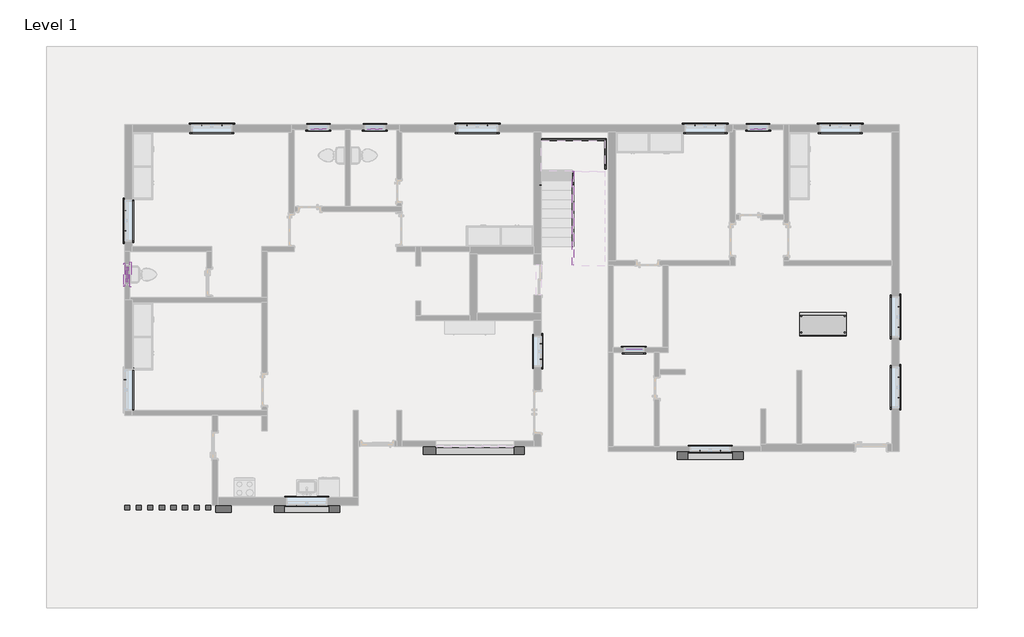
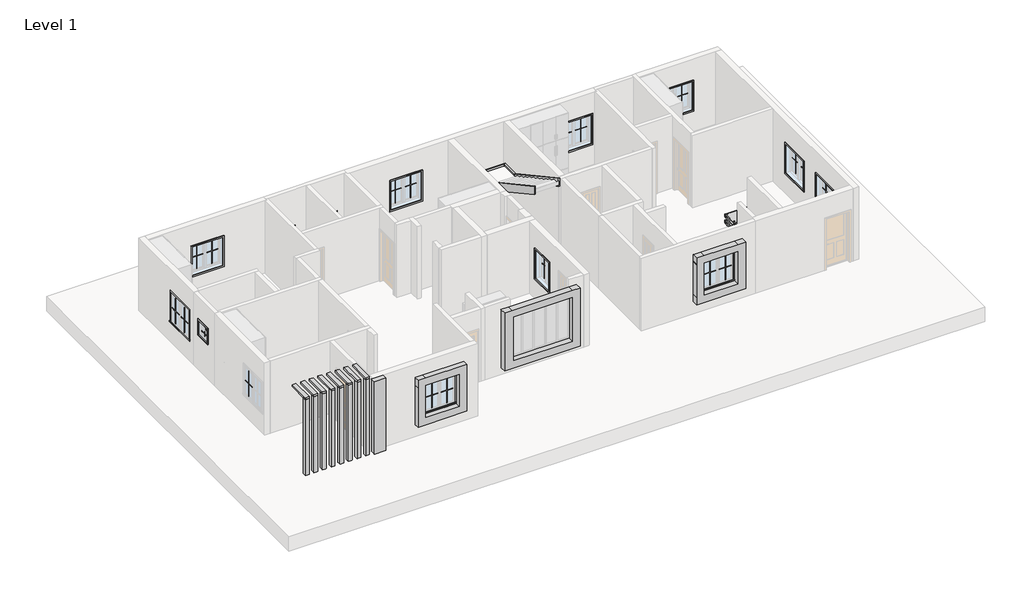
# One storey, part 3 of 3: 81 proxies, 7 members.
"""IFC4 building model written with IfcOpenShell, lengths in millimetres."""

from ifc_helpers import new_model, si_unit, frame, origin, place, context, project, spatial, polyline, outline, extrude, faceted_brep, transform, mapped, element, save
from components import generic_models_1_generic_models_1_a0d4ce11, generic_models_12_generic_models_1_bdc4cd0d, generic_models_13_generic_models_1_8ceb580d, generic_models_14_generic_models_1_67c994ca, generic_models_16_generic_models_16_6386461c, generic_models_17_generic_models_17_b8611751, generic_models_18_generic_models_18_97eb84db, generic_models_19_generic_models_19_60db133f, generic_models_2_generic_models_1_277b538b, generic_models_3_generic_models_1_ed787108, generic_models_4_generic_models_1_fab6a1cf, generic_models_5_generic_models_1_4439abc4, generic_models_6_generic_models_1_d5b3bf35, generic_models_7_generic_models_1_55103d6f, generic_models_8_generic_models_1_2d490598, modern_coffee_table_17989_modern_coffee_table_17989_d3a860c8, muntin_pattern_2x2_muntin_pattern_2x2_4dfeb3f3, muntin_pattern_2x2_muntin_pattern_2x2_e852a7e4, muntin_pattern_2x2_muntin_pattern_2x2_1acec82f, muntin_pattern_2x2_muntin_pattern_2x2_43d02eee, muntin_pattern_2x2_muntin_pattern_2x2_d17a704b, trim_window_exterior_flat_with_sill_7cfdd449, trim_window_exterior_flat_with_sill_e4b28ec3, trim_window_exterior_flat_with_sill_79c463f4, trim_window_interior_flat_picture_frame_f1e0b15b, trim_window_interior_flat_picture_frame_39ff4276, trim_window_interior_flat_picture_frame_0477b583

model = new_model("IFC4")

# Units and contexts
model_context = context("Model", 3, world=origin())
ifc_project = project(units=[si_unit("LENGTHUNIT", "METRE", prefix="MILLI")], contexts=[model_context])

# Site, building, storey
site = spatial("IfcSite", under=ifc_project)
building = spatial("IfcBuilding", under=site)
storey = spatial("IfcBuildingStorey", under=building, Name="Level 1", Elevation=0.0)

# Proxies
placement = place(None, origin())
generic_models_1_generic_models_1_shape = generic_models_1_generic_models_1_a0d4ce11(model_context)
element("IfcBuildingElementProxy", 1, Name="Generic Models 1 : Generic Models 1", ObjectType="Generic Models 1 : Generic Models 1", at=placement, inside=storey, context=model_context, shape_type="MappedRepresentation", body=[
    mapped(generic_models_1_generic_models_1_shape, transform((0.0, 0.0, 0.0), x_axis=(1.0, 0.0, 0.0), y_axis=(0.0, 1.0, 0.0), z_axis=(0.0, 0.0, 1.0))),
])
element("IfcBuildingElementProxy", 2, Name="Generic Models 10 : Generic Models 1", ObjectType="Generic Models 10 : Generic Models 1", at=placement, inside=storey, context=model_context, shape_type="MappedRepresentation", body=[
    mapped(generic_models_1_generic_models_1_shape, transform((0.0, 0.0, 0.0), x_axis=(1.0, 0.0, 0.0), y_axis=(0.0, 1.0, 0.0), z_axis=(0.0, 0.0, 1.0))),
])
element("IfcBuildingElementProxy", 3, Name="Generic Models 11 : Generic Models 1", ObjectType="Generic Models 11 : Generic Models 1", at=placement, inside=storey, context=model_context, shape_type="MappedRepresentation", body=[
    mapped(generic_models_1_generic_models_1_shape, transform((0.0, 0.0, 0.0), x_axis=(1.0, 0.0, 0.0), y_axis=(0.0, 1.0, 0.0), z_axis=(0.0, 0.0, 1.0))),
])
generic_models_12_generic_models_1_shape = generic_models_12_generic_models_1_bdc4cd0d(model_context)
element("IfcBuildingElementProxy", 4, Name="Generic Models 12 : Generic Models 1", ObjectType="Generic Models 12 : Generic Models 1", at=placement, inside=storey, context=model_context, shape_type="MappedRepresentation", body=[
    mapped(generic_models_12_generic_models_1_shape, transform((0.0, 0.0, 0.0), x_axis=(1.0, 0.0, 0.0), y_axis=(0.0, 1.0, 0.0), z_axis=(0.0, 0.0, 1.0))),
])
generic_models_13_generic_models_1_shape = generic_models_13_generic_models_1_8ceb580d(model_context)
element("IfcBuildingElementProxy", 5, Name="Generic Models 13 : Generic Models 1", ObjectType="Generic Models 13 : Generic Models 1", at=placement, inside=storey, context=model_context, shape_type="MappedRepresentation", body=[
    mapped(generic_models_13_generic_models_1_shape, transform((0.0, 0.0, 0.0), x_axis=(1.0, 0.0, 0.0), y_axis=(0.0, 1.0, 0.0), z_axis=(0.0, 0.0, 1.0))),
])
generic_models_14_generic_models_1_shape = generic_models_14_generic_models_1_67c994ca(model_context)
element("IfcBuildingElementProxy", 6, Name="Generic Models 14 : Generic Models 1", ObjectType="Generic Models 14 : Generic Models 1", at=placement, inside=storey, context=model_context, shape_type="MappedRepresentation", body=[
    mapped(generic_models_14_generic_models_1_shape, transform((0.0, 0.0, 0.0), x_axis=(1.0, 0.0, 0.0), y_axis=(0.0, 1.0, 0.0), z_axis=(0.0, 0.0, 1.0))),
])
generic_models_16_generic_models_16_shape = generic_models_16_generic_models_16_6386461c(model_context)
element("IfcBuildingElementProxy", 7, Name="Generic Models 16 : Generic Models 16", ObjectType="Generic Models 16 : Generic Models 16", at=placement, inside=storey, context=model_context, shape_type="MappedRepresentation", body=[
    mapped(generic_models_16_generic_models_16_shape, transform((0.0, 0.0, 0.0), x_axis=(1.0, 0.0, 0.0), y_axis=(0.0, 1.0, 0.0), z_axis=(0.0, 0.0, 1.0))),
])
generic_models_17_generic_models_17_shape = generic_models_17_generic_models_17_b8611751(model_context)
element("IfcBuildingElementProxy", 8, Name="Generic Models 17 : Generic Models 17", ObjectType="Generic Models 17 : Generic Models 17", at=placement, inside=storey, context=model_context, shape_type="MappedRepresentation", body=[
    mapped(generic_models_17_generic_models_17_shape, transform((0.0, 0.0, 0.0), x_axis=(1.0, 0.0, 0.0), y_axis=(0.0, 1.0, 0.0), z_axis=(0.0, 0.0, 1.0))),
])
generic_models_18_generic_models_18_shape = generic_models_18_generic_models_18_97eb84db(model_context)
element("IfcBuildingElementProxy", 9, Name="Generic Models 18 : Generic Models 18", ObjectType="Generic Models 18 : Generic Models 18", at=placement, inside=storey, context=model_context, shape_type="MappedRepresentation", body=[
    mapped(generic_models_18_generic_models_18_shape, transform((0.0, 0.0, 0.0), x_axis=(1.0, 0.0, 0.0), y_axis=(0.0, 1.0, 0.0), z_axis=(0.0, 0.0, 1.0))),
])
generic_models_19_generic_models_19_shape = generic_models_19_generic_models_19_60db133f(model_context)
element("IfcBuildingElementProxy", 10, Name="Generic Models 19 : Generic Models 19", ObjectType="Generic Models 19 : Generic Models 19", at=placement, inside=storey, context=model_context, shape_type="MappedRepresentation", body=[
    mapped(generic_models_19_generic_models_19_shape, transform((0.0, 0.0, 0.0), x_axis=(1.0, 0.0, 0.0), y_axis=(0.0, 1.0, 0.0), z_axis=(0.0, 0.0, 1.0))),
])
generic_models_2_generic_models_1_shape = generic_models_2_generic_models_1_277b538b(model_context)
element("IfcBuildingElementProxy", 11, Name="Generic Models 2 : Generic Models 1", ObjectType="Generic Models 2 : Generic Models 1", at=placement, inside=storey, context=model_context, shape_type="MappedRepresentation", body=[
    mapped(generic_models_2_generic_models_1_shape, transform((0.0, 0.0, 0.0), x_axis=(1.0, 0.0, 0.0), y_axis=(0.0, 1.0, 0.0), z_axis=(0.0, 0.0, 1.0))),
])
generic_models_3_generic_models_1_shape = generic_models_3_generic_models_1_ed787108(model_context)
element("IfcBuildingElementProxy", 12, Name="Generic Models 3 : Generic Models 1", ObjectType="Generic Models 3 : Generic Models 1", at=placement, inside=storey, context=model_context, shape_type="MappedRepresentation", body=[
    mapped(generic_models_3_generic_models_1_shape, transform((0.0, 0.0, 0.0), x_axis=(1.0, 0.0, 0.0), y_axis=(0.0, 1.0, 0.0), z_axis=(0.0, 0.0, 1.0))),
])
generic_models_4_generic_models_1_shape = generic_models_4_generic_models_1_fab6a1cf(model_context)
element("IfcBuildingElementProxy", 13, Name="Generic Models 4 : Generic Models 1", ObjectType="Generic Models 4 : Generic Models 1", at=placement, inside=storey, context=model_context, shape_type="MappedRepresentation", body=[
    mapped(generic_models_4_generic_models_1_shape, transform((0.0, 0.0, 0.0), x_axis=(1.0, 0.0, 0.0), y_axis=(0.0, 1.0, 0.0), z_axis=(0.0, 0.0, 1.0))),
])
generic_models_5_generic_models_1_shape = generic_models_5_generic_models_1_4439abc4(model_context)
element("IfcBuildingElementProxy", 14, Name="Generic Models 5 : Generic Models 1", ObjectType="Generic Models 5 : Generic Models 1", at=placement, inside=storey, context=model_context, shape_type="MappedRepresentation", body=[
    mapped(generic_models_5_generic_models_1_shape, transform((0.0, 0.0, 0.0), x_axis=(1.0, 0.0, 0.0), y_axis=(0.0, 1.0, 0.0), z_axis=(0.0, 0.0, 1.0))),
])
generic_models_6_generic_models_1_shape = generic_models_6_generic_models_1_d5b3bf35(model_context)
element("IfcBuildingElementProxy", 15, Name="Generic Models 6 : Generic Models 1", ObjectType="Generic Models 6 : Generic Models 1", at=placement, inside=storey, context=model_context, shape_type="MappedRepresentation", body=[
    mapped(generic_models_6_generic_models_1_shape, transform((0.0, 0.0, 0.0), x_axis=(1.0, 0.0, 0.0), y_axis=(0.0, 1.0, 0.0), z_axis=(0.0, 0.0, 1.0))),
])
generic_models_7_generic_models_1_shape = generic_models_7_generic_models_1_55103d6f(model_context)
element("IfcBuildingElementProxy", 16, Name="Generic Models 7 : Generic Models 1", ObjectType="Generic Models 7 : Generic Models 1", at=placement, inside=storey, context=model_context, shape_type="MappedRepresentation", body=[
    mapped(generic_models_7_generic_models_1_shape, transform((0.0, 0.0, 0.0), x_axis=(1.0, 0.0, 0.0), y_axis=(0.0, 1.0, 0.0), z_axis=(0.0, 0.0, 1.0))),
])
generic_models_8_generic_models_1_shape = generic_models_8_generic_models_1_2d490598(model_context)
element("IfcBuildingElementProxy", 17, Name="Generic Models 8 : Generic Models 1", ObjectType="Generic Models 8 : Generic Models 1", at=placement, inside=storey, context=model_context, shape_type="MappedRepresentation", body=[
    mapped(generic_models_8_generic_models_1_shape, transform((0.0, 0.0, 0.0), x_axis=(1.0, 0.0, 0.0), y_axis=(0.0, 1.0, 0.0), z_axis=(0.0, 0.0, 1.0))),
])
element("IfcBuildingElementProxy", 18, Name="Generic Models 9 : Generic Models 1", ObjectType="Generic Models 9 : Generic Models 1", at=placement, inside=storey, context=model_context, shape_type="MappedRepresentation", body=[
    mapped(generic_models_1_generic_models_1_shape, transform((0.0, 0.0, 0.0), x_axis=(1.0, 0.0, 0.0), y_axis=(0.0, 1.0, 0.0), z_axis=(0.0, 0.0, 1.0))),
])
modern_coffee_table_17989_modern_coffee_table_17989_shape = modern_coffee_table_17989_modern_coffee_table_17989_d3a860c8(model_context)
element("IfcBuildingElementProxy", 19, Name="Modern_Coffee_Table_17989 : Modern_Coffee_Table_17989", ObjectType="Modern_Coffee_Table_17989 : Modern_Coffee_Table_17989", at=placement, inside=storey, context=model_context, shape_type="MappedRepresentation", body=[
    mapped(modern_coffee_table_17989_modern_coffee_table_17989_shape, transform((8876.5549644, 263.8114998, 0.0), x_axis=(1.0, 0.0, 0.0), y_axis=(0.0, 1.0, 0.0), z_axis=(0.0, 0.0, 1.0))),
])
muntin_pattern_2x2_muntin_pattern_2x2_shape = muntin_pattern_2x2_muntin_pattern_2x2_4dfeb3f3(model_context)
element("IfcBuildingElementProxy", 20, Name="Muntin Pattern_2x2 : Muntin Pattern_2x2", ObjectType="Muntin Pattern_2x2 : Muntin Pattern_2x2", at=placement, inside=storey, context=model_context, shape_type="MappedRepresentation", body=[
    mapped(muntin_pattern_2x2_muntin_pattern_2x2_shape, transform((-9812.5661806, 5834.4476898, 984.25), x_axis=(1.0, 0.0, 0.0), y_axis=(0.0, 1.0, 0.0), z_axis=(0.0, 0.0, 1.0))),
])
element("IfcBuildingElementProxy", 21, Name="Muntin Pattern_2x2 : Muntin Pattern_2x2", ObjectType="Muntin Pattern_2x2 : Muntin Pattern_2x2", at=placement, inside=storey, context=model_context, shape_type="MappedRepresentation", body=[
    mapped(muntin_pattern_2x2_muntin_pattern_2x2_shape, transform((-1925.8661806, 5834.4476898, 984.25), x_axis=(1.0, 0.0, 0.0), y_axis=(0.0, 1.0, 0.0), z_axis=(0.0, 0.0, 1.0))),
])
element("IfcBuildingElementProxy", 22, Name="Muntin Pattern_2x2 : Muntin Pattern_2x2", ObjectType="Muntin Pattern_2x2 : Muntin Pattern_2x2", at=placement, inside=storey, context=model_context, shape_type="MappedRepresentation", body=[
    mapped(muntin_pattern_2x2_muntin_pattern_2x2_shape, transform((4843.2338194, 5834.4476898, 984.25), x_axis=(1.0, 0.0, 0.0), y_axis=(0.0, 1.0, 0.0), z_axis=(0.0, 0.0, 1.0))),
])
element("IfcBuildingElementProxy", 23, Name="Muntin Pattern_2x2 : Muntin Pattern_2x2", ObjectType="Muntin Pattern_2x2 : Muntin Pattern_2x2", at=placement, inside=storey, context=model_context, shape_type="MappedRepresentation", body=[
    mapped(muntin_pattern_2x2_muntin_pattern_2x2_shape, transform((8856.4338194, 5834.4476898, 984.25), x_axis=(1.0, 0.0, 0.0), y_axis=(0.0, 1.0, 0.0), z_axis=(0.0, 0.0, 1.0))),
])
element("IfcBuildingElementProxy", 24, Name="Muntin Pattern_2x2 : Muntin Pattern_2x2", ObjectType="Muntin Pattern_2x2 : Muntin Pattern_2x2", at=placement, inside=storey, context=model_context, shape_type="MappedRepresentation", body=[
    mapped(muntin_pattern_2x2_muntin_pattern_2x2_shape, transform((10902.7213194, 432.1851898, 984.25), x_axis=(0.0, -1.0, 0.0), y_axis=(1.0, 0.0, 0.0), z_axis=(0.0, 0.0, 1.0))),
])
element("IfcBuildingElementProxy", 25, Name="Muntin Pattern_2x2 : Muntin Pattern_2x2", ObjectType="Muntin Pattern_2x2 : Muntin Pattern_2x2", at=placement, inside=storey, context=model_context, shape_type="MappedRepresentation", body=[
    mapped(muntin_pattern_2x2_muntin_pattern_2x2_shape, transform((10902.7213194, -1663.3148102, 984.25), x_axis=(0.0, -1.0, 0.0), y_axis=(1.0, 0.0, 0.0), z_axis=(0.0, 0.0, 1.0))),
])
element("IfcBuildingElementProxy", 26, Name="Muntin Pattern_2x2 : Muntin Pattern_2x2", ObjectType="Muntin Pattern_2x2 : Muntin Pattern_2x2", at=placement, inside=storey, context=model_context, shape_type="MappedRepresentation", body=[
    mapped(muntin_pattern_2x2_muntin_pattern_2x2_shape, transform((5595.7088194, -3862.0023102, 984.25), x_axis=(-1.0, 0.0, 0.0), y_axis=(0.0, -1.0, 0.0), z_axis=(0.0, 0.0, 1.0))),
])
element("IfcBuildingElementProxy", 27, Name="Muntin Pattern_2x2 : Muntin Pattern_2x2", ObjectType="Muntin Pattern_2x2 : Muntin Pattern_2x2", at=placement, inside=storey, context=model_context, shape_type="MappedRepresentation", body=[
    mapped(muntin_pattern_2x2_muntin_pattern_2x2_shape, transform((-12090.6286806, 2683.2601898, 984.25), x_axis=(0.0, 1.0, 0.0), y_axis=(-1.0, 0.0, 0.0), z_axis=(0.0, 0.0, 1.0))),
])
element("IfcBuildingElementProxy", 28, Name="Muntin Pattern_2x2 : Muntin Pattern_2x2", ObjectType="Muntin Pattern_2x2 : Muntin Pattern_2x2", at=placement, inside=storey, context=model_context, shape_type="MappedRepresentation", body=[
    mapped(muntin_pattern_2x2_muntin_pattern_2x2_shape, transform((-6386.7411806, -5462.2023102, 984.25), x_axis=(-1.0, 0.0, 0.0), y_axis=(0.0, -1.0, 0.0), z_axis=(0.0, 0.0, 1.0))),
])
muntin_pattern_2x2_muntin_pattern_2x2_2_shape = muntin_pattern_2x2_muntin_pattern_2x2_e852a7e4(model_context)
element("IfcBuildingElementProxy", 29, Name="Muntin Pattern_2x2 : Muntin Pattern_2x2", ObjectType="Muntin Pattern_2x2 : Muntin Pattern_2x2", at=placement, inside=storey, context=model_context, shape_type="MappedRepresentation", body=[
    mapped(muntin_pattern_2x2_muntin_pattern_2x2_2_shape, transform((-9206.1411806, 5834.4476898, 984.25), x_axis=(-1.0, 0.0, 0.0), y_axis=(0.0, -1.0, 0.0), z_axis=(0.0, 0.0, 1.0))),
])
element("IfcBuildingElementProxy", 30, Name="Muntin Pattern_2x2 : Muntin Pattern_2x2", ObjectType="Muntin Pattern_2x2 : Muntin Pattern_2x2", at=placement, inside=storey, context=model_context, shape_type="MappedRepresentation", body=[
    mapped(muntin_pattern_2x2_muntin_pattern_2x2_2_shape, transform((-1319.4411806, 5834.4476898, 984.25), x_axis=(-1.0, 0.0, 0.0), y_axis=(0.0, -1.0, 0.0), z_axis=(0.0, 0.0, 1.0))),
])
element("IfcBuildingElementProxy", 31, Name="Muntin Pattern_2x2 : Muntin Pattern_2x2", ObjectType="Muntin Pattern_2x2 : Muntin Pattern_2x2", at=placement, inside=storey, context=model_context, shape_type="MappedRepresentation", body=[
    mapped(muntin_pattern_2x2_muntin_pattern_2x2_2_shape, transform((5449.6588194, 5834.4476898, 984.25), x_axis=(-1.0, 0.0, 0.0), y_axis=(0.0, -1.0, 0.0), z_axis=(0.0, 0.0, 1.0))),
])
element("IfcBuildingElementProxy", 32, Name="Muntin Pattern_2x2 : Muntin Pattern_2x2", ObjectType="Muntin Pattern_2x2 : Muntin Pattern_2x2", at=placement, inside=storey, context=model_context, shape_type="MappedRepresentation", body=[
    mapped(muntin_pattern_2x2_muntin_pattern_2x2_2_shape, transform((9462.8588194, 5834.4476898, 984.25), x_axis=(-1.0, 0.0, 0.0), y_axis=(0.0, -1.0, 0.0), z_axis=(0.0, 0.0, 1.0))),
])
element("IfcBuildingElementProxy", 33, Name="Muntin Pattern_2x2 : Muntin Pattern_2x2", ObjectType="Muntin Pattern_2x2 : Muntin Pattern_2x2", at=placement, inside=storey, context=model_context, shape_type="MappedRepresentation", body=[
    mapped(muntin_pattern_2x2_muntin_pattern_2x2_2_shape, transform((10902.7213194, -174.2398102, 984.25), x_axis=(0.0, 1.0, 0.0), y_axis=(-1.0, 0.0, 0.0), z_axis=(0.0, 0.0, 1.0))),
])
element("IfcBuildingElementProxy", 34, Name="Muntin Pattern_2x2 : Muntin Pattern_2x2", ObjectType="Muntin Pattern_2x2 : Muntin Pattern_2x2", at=placement, inside=storey, context=model_context, shape_type="MappedRepresentation", body=[
    mapped(muntin_pattern_2x2_muntin_pattern_2x2_2_shape, transform((10902.7213194, -2269.7398102, 984.25), x_axis=(0.0, 1.0, 0.0), y_axis=(-1.0, 0.0, 0.0), z_axis=(0.0, 0.0, 1.0))),
])
element("IfcBuildingElementProxy", 35, Name="Muntin Pattern_2x2 : Muntin Pattern_2x2", ObjectType="Muntin Pattern_2x2 : Muntin Pattern_2x2", at=placement, inside=storey, context=model_context, shape_type="MappedRepresentation", body=[
    mapped(muntin_pattern_2x2_muntin_pattern_2x2_2_shape, transform((-12090.6286806, -1739.5148102, 984.25), x_axis=(0.0, -1.0, 0.0), y_axis=(1.0, 0.0, 0.0), z_axis=(0.0, 0.0, 1.0))),
])
element("IfcBuildingElementProxy", 36, Name="Muntin Pattern_2x2 : Muntin Pattern_2x2", ObjectType="Muntin Pattern_2x2 : Muntin Pattern_2x2", at=placement, inside=storey, context=model_context, shape_type="MappedRepresentation", body=[
    mapped(muntin_pattern_2x2_muntin_pattern_2x2_2_shape, transform((4989.2838194, -3862.0023102, 984.25), x_axis=(1.0, 0.0, 0.0), y_axis=(0.0, 1.0, 0.0), z_axis=(0.0, 0.0, 1.0))),
])
element("IfcBuildingElementProxy", 37, Name="Muntin Pattern_2x2 : Muntin Pattern_2x2", ObjectType="Muntin Pattern_2x2 : Muntin Pattern_2x2", at=placement, inside=storey, context=model_context, shape_type="MappedRepresentation", body=[
    mapped(muntin_pattern_2x2_muntin_pattern_2x2_2_shape, transform((-12090.6286806, 3289.6851898, 984.25), x_axis=(0.0, -1.0, 0.0), y_axis=(1.0, 0.0, 0.0), z_axis=(0.0, 0.0, 1.0))),
])
element("IfcBuildingElementProxy", 38, Name="Muntin Pattern_2x2 : Muntin Pattern_2x2", ObjectType="Muntin Pattern_2x2 : Muntin Pattern_2x2", at=placement, inside=storey, context=model_context, shape_type="MappedRepresentation", body=[
    mapped(muntin_pattern_2x2_muntin_pattern_2x2_2_shape, transform((-6993.1661806, -5462.2023102, 984.25), x_axis=(1.0, 0.0, 0.0), y_axis=(0.0, 1.0, 0.0), z_axis=(0.0, 0.0, 1.0))),
])
muntin_pattern_2x2_muntin_pattern_2x2_3_shape = muntin_pattern_2x2_muntin_pattern_2x2_1acec82f(model_context)
element("IfcBuildingElementProxy", 39, Name="Muntin Pattern_2x2 : Muntin Pattern_2x2", ObjectType="Muntin Pattern_2x2 : Muntin Pattern_2x2", at=placement, inside=storey, context=model_context, shape_type="MappedRepresentation", body=[
    mapped(muntin_pattern_2x2_muntin_pattern_2x2_3_shape, transform((272.8213194, -672.7148102, 984.25), x_axis=(0.0, -1.0, 0.0), y_axis=(1.0, 0.0, 0.0), z_axis=(0.0, 0.0, 1.0))),
])
muntin_pattern_2x2_muntin_pattern_2x2_4_shape = muntin_pattern_2x2_muntin_pattern_2x2_43d02eee(model_context)
element("IfcBuildingElementProxy", 40, Name="Muntin Pattern_2x2 : Muntin Pattern_2x2", ObjectType="Muntin Pattern_2x2 : Muntin Pattern_2x2", at=placement, inside=storey, context=model_context, shape_type="MappedRepresentation", body=[
    mapped(muntin_pattern_2x2_muntin_pattern_2x2_4_shape, transform((272.8213194, -1126.7398102, 984.25), x_axis=(0.0, 1.0, 0.0), y_axis=(-1.0, 0.0, 0.0), z_axis=(0.0, 0.0, 1.0))),
])
muntin_pattern_2x2_muntin_pattern_2x2_5_shape = muntin_pattern_2x2_muntin_pattern_2x2_d17a704b(model_context)
element("IfcBuildingElementProxy", 41, Name="Muntin Pattern_2x2 : Muntin Pattern_2x2", ObjectType="Muntin Pattern_2x2 : Muntin Pattern_2x2", at=placement, inside=storey, context=model_context, shape_type="MappedRepresentation", body=[
    mapped(muntin_pattern_2x2_muntin_pattern_2x2_5_shape, transform((-11982.6786806, 1386.2726898, 1844.675), x_axis=(0.0, -1.0, 0.0), y_axis=(1.0, 0.0, 0.0), z_axis=(0.0, 0.0, 1.0))),
])
element("IfcBuildingElementProxy", 42, Name="Muntin Pattern_2x2 : Muntin Pattern_2x2", ObjectType="Muntin Pattern_2x2 : Muntin Pattern_2x2", at=placement, inside=storey, context=model_context, shape_type="MappedRepresentation", body=[
    mapped(muntin_pattern_2x2_muntin_pattern_2x2_5_shape, transform((-12027.1286806, 1386.2726898, 1600.2), x_axis=(0.0, -1.0, 0.0), y_axis=(1.0, 0.0, 0.0), z_axis=(0.0, 0.0, 1.0))),
])
element("IfcBuildingElementProxy", 43, Name="Muntin Pattern_2x2 : Muntin Pattern_2x2", ObjectType="Muntin Pattern_2x2 : Muntin Pattern_2x2", at=placement, inside=storey, context=model_context, shape_type="MappedRepresentation", body=[
    mapped(muntin_pattern_2x2_muntin_pattern_2x2_5_shape, transform((-6347.0536806, 5726.4976898, 1235.075), x_axis=(-1.0, 0.0, 0.0), y_axis=(0.0, -1.0, 0.0), z_axis=(0.0, 0.0, 1.0))),
])
element("IfcBuildingElementProxy", 44, Name="Muntin Pattern_2x2 : Muntin Pattern_2x2", ObjectType="Muntin Pattern_2x2 : Muntin Pattern_2x2", at=placement, inside=storey, context=model_context, shape_type="MappedRepresentation", body=[
    mapped(muntin_pattern_2x2_muntin_pattern_2x2_5_shape, transform((-6347.0536806, 5770.9476898, 990.6), x_axis=(-1.0, 0.0, 0.0), y_axis=(0.0, -1.0, 0.0), z_axis=(0.0, 0.0, 1.0))),
])
element("IfcBuildingElementProxy", 45, Name="Muntin Pattern_2x2 : Muntin Pattern_2x2", ObjectType="Muntin Pattern_2x2 : Muntin Pattern_2x2", at=placement, inside=storey, context=model_context, shape_type="MappedRepresentation", body=[
    mapped(muntin_pattern_2x2_muntin_pattern_2x2_5_shape, transform((-4670.6536806, 5726.4976898, 1235.075), x_axis=(-1.0, 0.0, 0.0), y_axis=(0.0, -1.0, 0.0), z_axis=(0.0, 0.0, 1.0))),
])
element("IfcBuildingElementProxy", 46, Name="Muntin Pattern_2x2 : Muntin Pattern_2x2", ObjectType="Muntin Pattern_2x2 : Muntin Pattern_2x2", at=placement, inside=storey, context=model_context, shape_type="MappedRepresentation", body=[
    mapped(muntin_pattern_2x2_muntin_pattern_2x2_5_shape, transform((-4670.6536806, 5770.9476898, 990.6), x_axis=(-1.0, 0.0, 0.0), y_axis=(0.0, -1.0, 0.0), z_axis=(0.0, 0.0, 1.0))),
])
element("IfcBuildingElementProxy", 47, Name="Muntin Pattern_2x2 : Muntin Pattern_2x2", ObjectType="Muntin Pattern_2x2 : Muntin Pattern_2x2", at=placement, inside=storey, context=model_context, shape_type="MappedRepresentation", body=[
    mapped(muntin_pattern_2x2_muntin_pattern_2x2_5_shape, transform((6721.2463194, 5726.4976898, 1235.075), x_axis=(-1.0, 0.0, 0.0), y_axis=(0.0, -1.0, 0.0), z_axis=(0.0, 0.0, 1.0))),
])
element("IfcBuildingElementProxy", 48, Name="Muntin Pattern_2x2 : Muntin Pattern_2x2", ObjectType="Muntin Pattern_2x2 : Muntin Pattern_2x2", at=placement, inside=storey, context=model_context, shape_type="MappedRepresentation", body=[
    mapped(muntin_pattern_2x2_muntin_pattern_2x2_5_shape, transform((6721.2463194, 5770.9476898, 990.6), x_axis=(-1.0, 0.0, 0.0), y_axis=(0.0, -1.0, 0.0), z_axis=(0.0, 0.0, 1.0))),
])
element("IfcBuildingElementProxy", 49, Name="Muntin Pattern_2x2 : Muntin Pattern_2x2", ObjectType="Muntin Pattern_2x2 : Muntin Pattern_2x2", at=placement, inside=storey, context=model_context, shape_type="MappedRepresentation", body=[
    mapped(muntin_pattern_2x2_muntin_pattern_2x2_5_shape, transform((3025.5463194, -820.3523102, 1235.075), x_axis=(1.0, 0.0, 0.0), y_axis=(0.0, 1.0, 0.0), z_axis=(0.0, 0.0, 1.0))),
])
element("IfcBuildingElementProxy", 50, Name="Muntin Pattern_2x2 : Muntin Pattern_2x2", ObjectType="Muntin Pattern_2x2 : Muntin Pattern_2x2", at=placement, inside=storey, context=model_context, shape_type="MappedRepresentation", body=[
    mapped(muntin_pattern_2x2_muntin_pattern_2x2_5_shape, transform((3025.5463194, -864.8023102, 990.6), x_axis=(1.0, 0.0, 0.0), y_axis=(0.0, 1.0, 0.0), z_axis=(0.0, 0.0, 1.0))),
])
trim_window_exterior_flat_with_sill_shape = trim_window_exterior_flat_with_sill_7cfdd449(model_context)
element("IfcBuildingElementProxy", 51, Name="Trim-Window-Exterior-Flat : with Sill", ObjectType="Trim-Window-Exterior-Flat : with Sill", at=placement, inside=storey, context=model_context, shape_type="MappedRepresentation", body=[
    mapped(trim_window_exterior_flat_with_sill_shape, transform((-9509.3536806, 5843.9726898, 2133.6), x_axis=(-1.0, 0.0, 0.0), y_axis=(0.0, 0.0, 1.0), z_axis=(0.0, 1.0, 0.0))),
])
element("IfcBuildingElementProxy", 52, Name="Trim-Window-Exterior-Flat : with Sill", ObjectType="Trim-Window-Exterior-Flat : with Sill", at=placement, inside=storey, context=model_context, shape_type="MappedRepresentation", body=[
    mapped(trim_window_exterior_flat_with_sill_shape, transform((-1622.6536806, 5843.9726898, 2133.6), x_axis=(-1.0, 0.0, 0.0), y_axis=(0.0, 0.0, 1.0), z_axis=(0.0, 1.0, 0.0))),
])
element("IfcBuildingElementProxy", 53, Name="Trim-Window-Exterior-Flat : with Sill", ObjectType="Trim-Window-Exterior-Flat : with Sill", at=placement, inside=storey, context=model_context, shape_type="MappedRepresentation", body=[
    mapped(trim_window_exterior_flat_with_sill_shape, transform((5146.4463194, 5843.9726898, 2133.6), x_axis=(-1.0, 0.0, 0.0), y_axis=(0.0, 0.0, 1.0), z_axis=(0.0, 1.0, 0.0))),
])
element("IfcBuildingElementProxy", 54, Name="Trim-Window-Exterior-Flat : with Sill", ObjectType="Trim-Window-Exterior-Flat : with Sill", at=placement, inside=storey, context=model_context, shape_type="MappedRepresentation", body=[
    mapped(trim_window_exterior_flat_with_sill_shape, transform((9159.6463194, 5843.9726898, 2133.6), x_axis=(-1.0, 0.0, 0.0), y_axis=(0.0, 0.0, 1.0), z_axis=(0.0, 1.0, 0.0))),
])
element("IfcBuildingElementProxy", 55, Name="Trim-Window-Exterior-Flat : with Sill", ObjectType="Trim-Window-Exterior-Flat : with Sill", at=placement, inside=storey, context=model_context, shape_type="MappedRepresentation", body=[
    mapped(trim_window_exterior_flat_with_sill_shape, transform((10912.2463194, 128.9726898, 2133.6), x_axis=(0.0, 1.0, 0.0), y_axis=(0.0, 0.0, 1.0), z_axis=(1.0, 0.0, 0.0))),
])
element("IfcBuildingElementProxy", 56, Name="Trim-Window-Exterior-Flat : with Sill", ObjectType="Trim-Window-Exterior-Flat : with Sill", at=placement, inside=storey, context=model_context, shape_type="MappedRepresentation", body=[
    mapped(trim_window_exterior_flat_with_sill_shape, transform((10912.2463194, -1966.5273102, 2133.6), x_axis=(0.0, 1.0, 0.0), y_axis=(0.0, 0.0, 1.0), z_axis=(1.0, 0.0, 0.0))),
])
element("IfcBuildingElementProxy", 57, Name="Trim-Window-Exterior-Flat : with Sill", ObjectType="Trim-Window-Exterior-Flat : with Sill", at=placement, inside=storey, context=model_context, shape_type="MappedRepresentation", body=[
    mapped(trim_window_exterior_flat_with_sill_shape, transform((5292.4963194, -3871.5273102, 2133.6), x_axis=(1.0, 0.0, 0.0), y_axis=(0.0, 0.0, 1.0), z_axis=(0.0, -1.0, 0.0))),
])
element("IfcBuildingElementProxy", 58, Name="Trim-Window-Exterior-Flat : with Sill", ObjectType="Trim-Window-Exterior-Flat : with Sill", at=placement, inside=storey, context=model_context, shape_type="MappedRepresentation", body=[
    mapped(trim_window_exterior_flat_with_sill_shape, transform((-12100.1536806, 2986.4726898, 2133.6), x_axis=(0.0, -1.0, 0.0), y_axis=(0.0, 0.0, 1.0), z_axis=(-1.0, 0.0, 0.0))),
])
element("IfcBuildingElementProxy", 59, Name="Trim-Window-Exterior-Flat : with Sill", ObjectType="Trim-Window-Exterior-Flat : with Sill", at=placement, inside=storey, context=model_context, shape_type="MappedRepresentation", body=[
    mapped(trim_window_exterior_flat_with_sill_shape, transform((-6689.9536806, -5471.7273102, 2133.6), x_axis=(1.0, 0.0, 0.0), y_axis=(0.0, 0.0, 1.0), z_axis=(0.0, -1.0, 0.0))),
])
trim_window_exterior_flat_with_sill_2_shape = trim_window_exterior_flat_with_sill_e4b28ec3(model_context)
element("IfcBuildingElementProxy", 60, Name="Trim-Window-Exterior-Flat : with Sill", ObjectType="Trim-Window-Exterior-Flat : with Sill", at=placement, inside=storey, context=model_context, shape_type="MappedRepresentation", body=[
    mapped(trim_window_exterior_flat_with_sill_2_shape, transform((282.3463194, -899.7273102, 2133.6), x_axis=(0.0, 1.0, 0.0), y_axis=(0.0, 0.0, 1.0), z_axis=(1.0, 0.0, 0.0))),
])
trim_window_exterior_flat_with_sill_3_shape = trim_window_exterior_flat_with_sill_79c463f4(model_context)
element("IfcBuildingElementProxy", 61, Name="Trim-Window-Exterior-Flat : with Sill", ObjectType="Trim-Window-Exterior-Flat : with Sill", at=placement, inside=storey, context=model_context, shape_type="MappedRepresentation", body=[
    mapped(trim_window_exterior_flat_with_sill_3_shape, transform((-11947.7536806, 1386.2726898, 2120.9), x_axis=(0.0, 1.0, 0.0), y_axis=(0.0, 0.0, 1.0), z_axis=(1.0, 0.0, 0.0))),
])
element("IfcBuildingElementProxy", 62, Name="Trim-Window-Exterior-Flat : with Sill", ObjectType="Trim-Window-Exterior-Flat : with Sill", at=placement, inside=storey, context=model_context, shape_type="MappedRepresentation", body=[
    mapped(trim_window_exterior_flat_with_sill_3_shape, transform((-6347.0536806, 5691.5726898, 1511.3), x_axis=(1.0, 0.0, 0.0), y_axis=(0.0, 0.0, 1.0), z_axis=(0.0, -1.0, 0.0))),
])
element("IfcBuildingElementProxy", 63, Name="Trim-Window-Exterior-Flat : with Sill", ObjectType="Trim-Window-Exterior-Flat : with Sill", at=placement, inside=storey, context=model_context, shape_type="MappedRepresentation", body=[
    mapped(trim_window_exterior_flat_with_sill_3_shape, transform((-4670.6536806, 5691.5726898, 1511.3), x_axis=(1.0, 0.0, 0.0), y_axis=(0.0, 0.0, 1.0), z_axis=(0.0, -1.0, 0.0))),
])
element("IfcBuildingElementProxy", 64, Name="Trim-Window-Exterior-Flat : with Sill", ObjectType="Trim-Window-Exterior-Flat : with Sill", at=placement, inside=storey, context=model_context, shape_type="MappedRepresentation", body=[
    mapped(trim_window_exterior_flat_with_sill_3_shape, transform((6721.2463194, 5691.5726898, 1511.3), x_axis=(1.0, 0.0, 0.0), y_axis=(0.0, 0.0, 1.0), z_axis=(0.0, -1.0, 0.0))),
])
element("IfcBuildingElementProxy", 65, Name="Trim-Window-Exterior-Flat : with Sill", ObjectType="Trim-Window-Exterior-Flat : with Sill", at=placement, inside=storey, context=model_context, shape_type="MappedRepresentation", body=[
    mapped(trim_window_exterior_flat_with_sill_3_shape, transform((3025.5463194, -785.4273102, 1511.3), x_axis=(-1.0, 0.0, 0.0), y_axis=(0.0, 0.0, 1.0), z_axis=(0.0, 1.0, 0.0))),
])
trim_window_interior_flat_picture_frame_shape = trim_window_interior_flat_picture_frame_f1e0b15b(model_context)
element("IfcBuildingElementProxy", 66, Name="Trim-Window-Interior-Flat : Picture Frame", ObjectType="Trim-Window-Interior-Flat : Picture Frame", at=placement, inside=storey, context=model_context, shape_type="MappedRepresentation", body=[
    mapped(trim_window_interior_flat_picture_frame_shape, transform((-9509.3536806, 5615.3726898, 2133.6), x_axis=(1.0, 0.0, 0.0), y_axis=(0.0, 0.0, 1.0), z_axis=(0.0, -1.0, 0.0))),
])
element("IfcBuildingElementProxy", 67, Name="Trim-Window-Interior-Flat : Picture Frame", ObjectType="Trim-Window-Interior-Flat : Picture Frame", at=placement, inside=storey, context=model_context, shape_type="MappedRepresentation", body=[
    mapped(trim_window_interior_flat_picture_frame_shape, transform((-1622.6536806, 5615.3726898, 2133.6), x_axis=(1.0, 0.0, 0.0), y_axis=(0.0, 0.0, 1.0), z_axis=(0.0, -1.0, 0.0))),
])
element("IfcBuildingElementProxy", 68, Name="Trim-Window-Interior-Flat : Picture Frame", ObjectType="Trim-Window-Interior-Flat : Picture Frame", at=placement, inside=storey, context=model_context, shape_type="MappedRepresentation", body=[
    mapped(trim_window_interior_flat_picture_frame_shape, transform((5146.4463194, 5615.3726898, 2133.6), x_axis=(1.0, 0.0, 0.0), y_axis=(0.0, 0.0, 1.0), z_axis=(0.0, -1.0, 0.0))),
])
element("IfcBuildingElementProxy", 69, Name="Trim-Window-Interior-Flat : Picture Frame", ObjectType="Trim-Window-Interior-Flat : Picture Frame", at=placement, inside=storey, context=model_context, shape_type="MappedRepresentation", body=[
    mapped(trim_window_interior_flat_picture_frame_shape, transform((9159.6463194, 5615.3726898, 2133.6), x_axis=(1.0, 0.0, 0.0), y_axis=(0.0, 0.0, 1.0), z_axis=(0.0, -1.0, 0.0))),
])
element("IfcBuildingElementProxy", 70, Name="Trim-Window-Interior-Flat : Picture Frame", ObjectType="Trim-Window-Interior-Flat : Picture Frame", at=placement, inside=storey, context=model_context, shape_type="MappedRepresentation", body=[
    mapped(trim_window_interior_flat_picture_frame_shape, transform((10683.6463194, 128.9726898, 2133.6), x_axis=(0.0, -1.0, 0.0), y_axis=(0.0, 0.0, 1.0), z_axis=(-1.0, 0.0, 0.0))),
])
element("IfcBuildingElementProxy", 71, Name="Trim-Window-Interior-Flat : Picture Frame", ObjectType="Trim-Window-Interior-Flat : Picture Frame", at=placement, inside=storey, context=model_context, shape_type="MappedRepresentation", body=[
    mapped(trim_window_interior_flat_picture_frame_shape, transform((10683.6463194, -1966.5273102, 2133.6), x_axis=(0.0, -1.0, 0.0), y_axis=(0.0, 0.0, 1.0), z_axis=(-1.0, 0.0, 0.0))),
])
element("IfcBuildingElementProxy", 72, Name="Trim-Window-Interior-Flat : Picture Frame", ObjectType="Trim-Window-Interior-Flat : Picture Frame", at=placement, inside=storey, context=model_context, shape_type="MappedRepresentation", body=[
    mapped(trim_window_interior_flat_picture_frame_shape, transform((-11871.5536806, -2042.7273102, 2133.6), x_axis=(0.0, 1.0, 0.0), y_axis=(0.0, 0.0, 1.0), z_axis=(1.0, 0.0, 0.0))),
])
element("IfcBuildingElementProxy", 73, Name="Trim-Window-Interior-Flat : Picture Frame", ObjectType="Trim-Window-Interior-Flat : Picture Frame", at=placement, inside=storey, context=model_context, shape_type="MappedRepresentation", body=[
    mapped(trim_window_interior_flat_picture_frame_shape, transform((5292.4963194, -3719.1273102, 2133.6), x_axis=(-1.0, 0.0, 0.0), y_axis=(0.0, 0.0, 1.0), z_axis=(0.0, 1.0, 0.0))),
])
element("IfcBuildingElementProxy", 74, Name="Trim-Window-Interior-Flat : Picture Frame", ObjectType="Trim-Window-Interior-Flat : Picture Frame", at=placement, inside=storey, context=model_context, shape_type="MappedRepresentation", body=[
    mapped(trim_window_interior_flat_picture_frame_shape, transform((-11871.5536806, 2986.4726898, 2133.6), x_axis=(0.0, 1.0, 0.0), y_axis=(0.0, 0.0, 1.0), z_axis=(1.0, 0.0, 0.0))),
])
element("IfcBuildingElementProxy", 75, Name="Trim-Window-Interior-Flat : Picture Frame", ObjectType="Trim-Window-Interior-Flat : Picture Frame", at=placement, inside=storey, context=model_context, shape_type="MappedRepresentation", body=[
    mapped(trim_window_interior_flat_picture_frame_shape, transform((-6689.9536806, -5243.1273102, 2133.6), x_axis=(-1.0, 0.0, 0.0), y_axis=(0.0, 0.0, 1.0), z_axis=(0.0, 1.0, 0.0))),
])
trim_window_interior_flat_picture_frame_2_shape = trim_window_interior_flat_picture_frame_39ff4276(model_context)
element("IfcBuildingElementProxy", 76, Name="Trim-Window-Interior-Flat : Picture Frame", ObjectType="Trim-Window-Interior-Flat : Picture Frame", at=placement, inside=storey, context=model_context, shape_type="MappedRepresentation", body=[
    mapped(trim_window_interior_flat_picture_frame_2_shape, transform((53.7463194, -899.7273102, 2133.6), x_axis=(0.0, -1.0, 0.0), y_axis=(0.0, 0.0, 1.0), z_axis=(-1.0, 0.0, 0.0))),
])
trim_window_interior_flat_picture_frame_3_shape = trim_window_interior_flat_picture_frame_0477b583(model_context)
element("IfcBuildingElementProxy", 77, Name="Trim-Window-Interior-Flat : Picture Frame", ObjectType="Trim-Window-Interior-Flat : Picture Frame", at=placement, inside=storey, context=model_context, shape_type="MappedRepresentation", body=[
    mapped(trim_window_interior_flat_picture_frame_3_shape, transform((-12100.1536806, 1386.2726898, 2120.9), x_axis=(0.0, -1.0, 0.0), y_axis=(0.0, 0.0, 1.0), z_axis=(-1.0, 0.0, 0.0))),
])
element("IfcBuildingElementProxy", 78, Name="Trim-Window-Interior-Flat : Picture Frame", ObjectType="Trim-Window-Interior-Flat : Picture Frame", at=placement, inside=storey, context=model_context, shape_type="MappedRepresentation", body=[
    mapped(trim_window_interior_flat_picture_frame_3_shape, transform((-6347.0536806, 5843.9726898, 1511.3), x_axis=(-1.0, 0.0, 0.0), y_axis=(0.0, 0.0, 1.0), z_axis=(0.0, 1.0, 0.0))),
])
element("IfcBuildingElementProxy", 79, Name="Trim-Window-Interior-Flat : Picture Frame", ObjectType="Trim-Window-Interior-Flat : Picture Frame", at=placement, inside=storey, context=model_context, shape_type="MappedRepresentation", body=[
    mapped(trim_window_interior_flat_picture_frame_3_shape, transform((-4670.6536806, 5843.9726898, 1511.3), x_axis=(-1.0, 0.0, 0.0), y_axis=(0.0, 0.0, 1.0), z_axis=(0.0, 1.0, 0.0))),
])
element("IfcBuildingElementProxy", 80, Name="Trim-Window-Interior-Flat : Picture Frame", ObjectType="Trim-Window-Interior-Flat : Picture Frame", at=placement, inside=storey, context=model_context, shape_type="MappedRepresentation", body=[
    mapped(trim_window_interior_flat_picture_frame_3_shape, transform((6721.2463194, 5843.9726898, 1511.3), x_axis=(-1.0, 0.0, 0.0), y_axis=(0.0, 0.0, 1.0), z_axis=(0.0, 1.0, 0.0))),
])
element("IfcBuildingElementProxy", 81, Name="Trim-Window-Interior-Flat : Picture Frame", ObjectType="Trim-Window-Interior-Flat : Picture Frame", at=placement, inside=storey, context=model_context, shape_type="MappedRepresentation", body=[
    mapped(trim_window_interior_flat_picture_frame_3_shape, transform((3025.5463194, -937.8273102, 1511.3), x_axis=(1.0, 0.0, 0.0), y_axis=(0.0, 0.0, 1.0), z_axis=(0.0, -1.0, 0.0))),
])

# Members
element("IfcMember", 82, ObjectType="Stringer - 2\" Width", at=placement, inside=storey, context=model_context, shape_type="SweptSolid", body=[
    extrude(outline(polyline([(2224.4726898, 0.0), (2224.4726898, 206.7436667), (4499.7426342, 1447.8), (4577.4648098, 1143.0), (2481.9648098, 0.0), (2224.4726898, 0.0)])), frame((231.5463194, 0.0, 0.0), z_axis=(1.0, 0.0, 0.0), x_axis=(0.0, 1.0, 0.0)), (0.0, 0.0, 1.0), 50.8),
])
element("IfcMember", 83, ObjectType="Stringer - 2\" Width", at=placement, inside=storey, context=model_context, shape_type="SweptSolid", body=[
    extrude(outline(polyline([(2224.4726898, 0.0), (2224.4726898, 206.7436667), (4408.8726898, 1398.2345758), (4408.8726898, 1051.0406619), (2481.9648098, 0.0), (2224.4726898, 0.0)])), frame((1196.7463194, 0.0, 0.0), z_axis=(1.0, 0.0, 0.0), x_axis=(0.0, 1.0, 0.0)), (0.0, 0.0, 1.0), 50.8),
])
element("IfcMember", 84, ObjectType="Stringer - 2\" Width", at=placement, inside=storey, context=model_context, shape_type="SweptSolid", body=[
    extrude(outline(polyline([(4699.0027455, 1447.8), (4621.2805699, 1143.0), (1665.6726898, 2755.1497528), (1665.6726898, 3102.3436667), (4699.0027455, 1447.8)])), frame((2161.9463194, 0.0, 0.0), z_axis=(1.0, 0.0, 0.0), x_axis=(0.0, 1.0, 0.0)), (0.0, 0.0, 1.0), 50.8),
])
element("IfcMember", 85, ObjectType="Stringer - 2\" Width", at=placement, inside=storey, context=model_context, shape_type="SweptSolid", body=[
    extrude(outline(polyline([(4459.6726898, 1578.3436667), (4459.6726898, 1231.1497528), (1665.6726898, 2755.1497528), (1665.6726898, 3102.3436667), (4459.6726898, 1578.3436667)])), frame((1196.7463194, 0.0, 0.0), z_axis=(1.0, 0.0, 0.0), x_axis=(0.0, 1.0, 0.0)), (0.0, 0.0, 1.0), 50.8),
])
element("IfcMember", 86, ObjectType="Stringer - 2\" Width", at=placement, inside=storey, context=model_context, shape_type="Brep", body=[
    faceted_brep([(2161.9463194, 4699.0027455, 1447.8), (2212.7463194, 4699.0027455, 1447.8), (2212.7463194, 5424.8726898, 1447.8), (2161.9463194, 5374.0726898, 1447.8), (2161.9463194, 4621.2805699, 1143.0), (2161.9463194, 5374.0726898, 1143.0), (2212.7463194, 4621.2805699, 1143.0), (2212.7463194, 5424.8726898, 1143.0)], [[[0, 1, 2, 3]], [[4, 0, 3, 5]], [[6, 4, 5, 7]], [[1, 6, 7, 2]], [[1, 0, 4, 6]], [[2, 7, 5, 3]]]),
])
element("IfcMember", 87, ObjectType="Stringer - 2\" Width", at=placement, inside=storey, context=model_context, shape_type="SweptSolid", body=[
    extrude(outline(polyline([(2212.7463194, 5424.8726898), (2161.9463194, 5374.0726898), (282.3463194, 5374.0726898), (231.5463194, 5424.8726898), (2212.7463194, 5424.8726898)])), frame((0.0, 0.0, 1143.0), z_axis=(0.0, 0.0, 1.0), x_axis=(1.0, 0.0, 0.0)), (0.0, 0.0, 1.0), 304.8),
])
element("IfcMember", 88, ObjectType="Stringer - 2\" Width", at=placement, inside=storey, context=model_context, shape_type="Brep", body=[
    faceted_brep([(282.3463194, 5374.0726898, 1447.8), (231.5463194, 5424.8726898, 1447.8), (231.5463194, 4499.7426342, 1447.8), (282.3463194, 4499.7426342, 1447.8), (282.3463194, 5374.0726898, 1143.0), (282.3463194, 4577.4648098, 1143.0), (231.5463194, 5424.8726898, 1143.0), (231.5463194, 4577.4648098, 1143.0)], [[[0, 1, 2, 3]], [[4, 0, 3, 5]], [[6, 4, 5, 7]], [[1, 6, 7, 2]], [[1, 0, 4, 6]], [[2, 7, 5, 3]]]),
])

save(model, "model.ifc")

# Revit data of these elements
# Type "Modern_Coffee_Table_17989 : Modern_Coffee_Table_17989"
#   Default Elevation = 0
# Type "Muntin Pattern_2x2 : Muntin Pattern_2x2"
#   Width [instance default] = 4' - 0"
#   Thickness = 0' - 0 1/2"
#   Height [instance default] = 4' - 0"
#   Distance = 0' - 0 3/4"
#   Interior Material [instance default] = none
#   Exterior Material [instance default] = none
#   Default Elevation = 0
# Type "Trim-Window-Exterior-Flat : with Sill"
#   Trim Width = 0' - 2 1/4"
#   Trim Thickness_Picture Frame = 0' - 1 1/4"
#   Trim Thickness_with Sill = 0' - 0 3/4"
#   Sill Thickness = 0' - 1 1/4"
#   Opening Width [instance default] = 2' - 0"
#   Opening Height [instance default] = 3' - 0"
#   Default Elevation = 4' - 0"
#   Sill = yes
#   Picture Frame = no
#   Trim Material [instance default] = none
# Type "Trim-Window-Interior-Flat : Picture Frame"
#   Trim Thickness_Picture Frame = 0' - 1 1/4"
#   Trim Width = 0' - 2 1/4"
#   Trim Thickness_with Sill = 0' - 0 3/4"
#   Sill Thickness = 0' - 1 1/4"
#   Opening Width [instance default] = 2' - 0"
#   Opening Height [instance default] = 3' - 0"
#   Default Elevation = 4' - 0"
#   Sill = no
#   Picture Frame = yes
#   Trim Material [instance default] = none
# Element 1 (IfcBuildingElementProxy, "Generic Models 1 : Generic Models 1")
#   Phase Created = New Construction
#   Materials on its faces: "exterior wall"
# Element 2 (IfcBuildingElementProxy, "Generic Models 10 : Generic Models 1")
#   Phase Created = New Construction
# Element 3 (IfcBuildingElementProxy, "Generic Models 11 : Generic Models 1")
#   Phase Created = New Construction
# Element 4 (IfcBuildingElementProxy, "Generic Models 12 : Generic Models 1")
#   Phase Created = New Construction
#   Materials on its faces: "exterior wall"
# Element 5 (IfcBuildingElementProxy, "Generic Models 13 : Generic Models 1")
#   Phase Created = New Construction
# Element 6 (IfcBuildingElementProxy, "Generic Models 14 : Generic Models 1")
#   Phase Created = New Construction
# Element 7 (IfcBuildingElementProxy, "Generic Models 16 : Generic Models 16")
#   Phase Created = New Construction
#   Materials on its faces: "exterior wall"
# Element 8 (IfcBuildingElementProxy, "Generic Models 17 : Generic Models 17")
#   Phase Created = New Construction
#   Materials on its faces: "exterior wall", "wall"
# Element 9 (IfcBuildingElementProxy, "Generic Models 18 : Generic Models 18")
#   Phase Created = New Construction
#   Materials on its faces: "exterior wall"
# Element 10 (IfcBuildingElementProxy, "Generic Models 19 : Generic Models 19")
#   Phase Created = New Construction
#   Materials on its faces: "exterior wall"
# Element 11 (IfcBuildingElementProxy, "Generic Models 2 : Generic Models 1")
#   Phase Created = New Construction
# Element 12 (IfcBuildingElementProxy, "Generic Models 3 : Generic Models 1")
#   Phase Created = New Construction
# Element 13 (IfcBuildingElementProxy, "Generic Models 4 : Generic Models 1")
#   Phase Created = New Construction
# Element 14 (IfcBuildingElementProxy, "Generic Models 5 : Generic Models 1")
#   Phase Created = New Construction
# Element 15 (IfcBuildingElementProxy, "Generic Models 6 : Generic Models 1")
#   Phase Created = New Construction
# Element 16 (IfcBuildingElementProxy, "Generic Models 7 : Generic Models 1")
#   Phase Created = New Construction
# Element 17 (IfcBuildingElementProxy, "Generic Models 8 : Generic Models 1")
#   Phase Created = New Construction
# Element 18 (IfcBuildingElementProxy, "Generic Models 9 : Generic Models 1")
#   Phase Created = New Construction
# Element 19 (IfcBuildingElementProxy, "Modern_Coffee_Table_17989 : Modern_Coffee_Table_17989")
#   Phase Created = New Construction
#   Materials on its faces: "1 WOOD", "1 Glass", "1 Metal"
# Elements 20, 21, 22, 23, 24, 25, 26, 27, 28, 29, 30, 31, 32, 33, 34, 35, 36, 37, 38 (IfcBuildingElementProxy, "Muntin Pattern_2x2 : Muntin Pattern_2x2")
#   Width = 1' - 6 5/8"
#   Height = 3' - 6 1/2"
#   Interior Material = Wood - Stained
#   Exterior Material = Clad - White
#   Phase Created = New Construction
#   Materials on its faces: "Clad - White", "Wood - Stained"
# Elements 39, 40 (IfcBuildingElementProxy, "Muntin Pattern_2x2 : Muntin Pattern_2x2")
#   Width = 1' - 0 5/8"
#   Height = 3' - 6 1/2"
#   Interior Material = Wood - Stained
#   Exterior Material = Clad - White
#   Phase Created = New Construction
#   Materials on its faces: "Clad - White", "Wood - Stained"
# Elements 41, 42, 43, 44, 45, 46, 47, 48, 49, 50 (IfcBuildingElementProxy, "Muntin Pattern_2x2 : Muntin Pattern_2x2")
#   Width = 1' - 6"
#   Height = 0' - 7 7/8"
#   Interior Material = Wood - Stained
#   Exterior Material = Clad - White
#   Phase Created = New Construction
#   Materials on its faces: "Clad - White", "Wood - Stained"
# Elements 51, 52, 53, 54, 55, 56, 57, 58, 59 (IfcBuildingElementProxy, "Trim-Window-Exterior-Flat : with Sill")
#   Opening Width = 4' - 0"
#   Opening Height = 4' - 0"
#   Trim Material = Clad - White
#   Phase Created = New Construction
#   Materials on its faces: "Clad - White"
# Element 60 (IfcBuildingElementProxy, "Trim-Window-Exterior-Flat : with Sill")
#   Opening Width = 3' - 0"
#   Opening Height = 4' - 0"
#   Trim Material = Clad - White
#   Phase Created = New Construction
#   Materials on its faces: "Clad - White"
# Elements 61, 62, 63, 64, 65 (IfcBuildingElementProxy, "Trim-Window-Exterior-Flat : with Sill")
#   Opening Width = 2' - 0"
#   Opening Height = 1' - 11 1/2"
#   Trim Material = Clad - White
#   Phase Created = New Construction
#   Materials on its faces: "Clad - White"
# Elements 66, 67, 68, 69, 70, 71, 72, 73, 74, 75 (IfcBuildingElementProxy, "Trim-Window-Interior-Flat : Picture Frame")
#   Opening Width = 4' - 0"
#   Opening Height = 4' - 0"
#   Trim Material = Wood - Stained
#   Phase Created = New Construction
#   Materials on its faces: "Wood - Stained"
# Element 76 (IfcBuildingElementProxy, "Trim-Window-Interior-Flat : Picture Frame")
#   Opening Width = 3' - 0"
#   Opening Height = 4' - 0"
#   Trim Material = Wood - Stained
#   Phase Created = New Construction
#   Materials on its faces: "Wood - Stained"
# Elements 77, 78, 79, 80, 81 (IfcBuildingElementProxy, "Trim-Window-Interior-Flat : Picture Frame")
#   Opening Width = 2' - 0"
#   Opening Height = 1' - 11 1/2"
#   Trim Material = Wood - Stained
#   Phase Created = New Construction
#   Materials on its faces: "Wood - Stained"
# Elements 82, 83, 84, 85, 86, 87, 88 (IfcMember, "Stringer - 2\" Width")
#   Phase Created = New Construction
# Materials
#   "exterior wall": class "Generic", colour RGB 215 217 121, transparency 0, Cost = 0
#   "wall": class "Generic", colour RGB 127 127 127, transparency 0, Cost = 0
#   "1 WOOD": colour RGB 32 25 15, transparency 0
#   "1 Glass": class "Glass", colour RGB 236 240 239, transparency 0.85, Cost = 0
#   "1 Metal": class "Glass", colour RGB 244 244 244, transparency 0, Cost = 0
#   "Clad - White": class "Wood", colour RGB 242 242 238, transparency 0, Cost = 0
#   "Wood - Stained": class "Wood", colour RGB 224 178 126, transparency 0, Cost = 0
